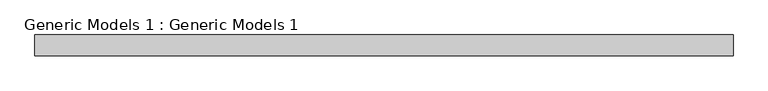
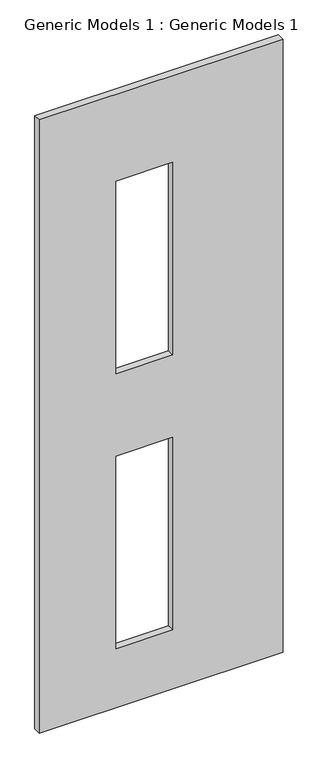
"""IFC4 building model written with IfcOpenShell, lengths in millimetres: proxy geometry, Generic Models 1 : Generic Models 1."""

from ifc_helpers import new_model, si_unit, frame, origin, place, context, project, spatial, polyline, outline, extrude, source, transform, mapped, element, save


def generic_models_1_generic_models_1_a9dcc39e(model_context):
    return source(origin(), model_context, "Body", "SweptSolid", [
        extrude(outline(polyline([(13594.3190306, -10192.3456086), (13594.3190306, -15310.4456086), (0.0, -15310.4456086), (0.0, -10192.3456086), (13594.3190306, -10192.3456086)]), holes=[polyline([(11668.0, -12503.7456086), (7400.8, -12503.7456086), (7400.8, -13697.5456086), (11668.0, -13697.5456086), (11668.0, -12503.7456086)]), polyline([(5572.0, -12503.7456086), (1304.8, -12503.7456086), (1304.8, -13697.5456086), (5572.0, -13697.5456086), (5572.0, -12503.7456086)])]), frame((0.0, -11268.8679047, 0.0), z_axis=(0.0, 1.0, 0.0), x_axis=(0.0, 0.0, 1.0)), (0.0, 0.0, 1.0), 152.4),
    ])


if __name__ == "__main__":
    model = new_model("IFC4")
    model_context = context("Model", 3, world=origin())
    ifc_project = project(units=[si_unit("LENGTHUNIT", "METRE", prefix="MILLI")], contexts=[model_context])
    site = spatial("IfcSite", under=ifc_project)
    building = spatial("IfcBuilding", under=site)
    placement = place(None, origin())
    generic_models_1_generic_models_1_shape = generic_models_1_generic_models_1_a9dcc39e(model_context)
    element("IfcBuildingElementProxy", 1, Name="Generic Models 1 : Generic Models 1", ObjectType="Generic Models 1 : Generic Models 1", at=placement, inside=building, context=model_context, shape_type="MappedRepresentation", body=[
        mapped(generic_models_1_generic_models_1_shape, transform((0.0, 0.0, 0.0), x_axis=(1.0, 0.0, 0.0), y_axis=(0.0, 1.0, 0.0), z_axis=(0.0, 0.0, 1.0))),
    ])
    save(model, "model.ifc")

# Revit data of these elements
# Element 1 (IfcBuildingElementProxy, "Generic Models 1 : Generic Models 1")
#   Materials on its faces: "WALL ACCENT 6\""
# Materials
#   "WALL ACCENT 6\"": class "Generic", colour RGB 120 120 120, transparency 0, Cost = 0
